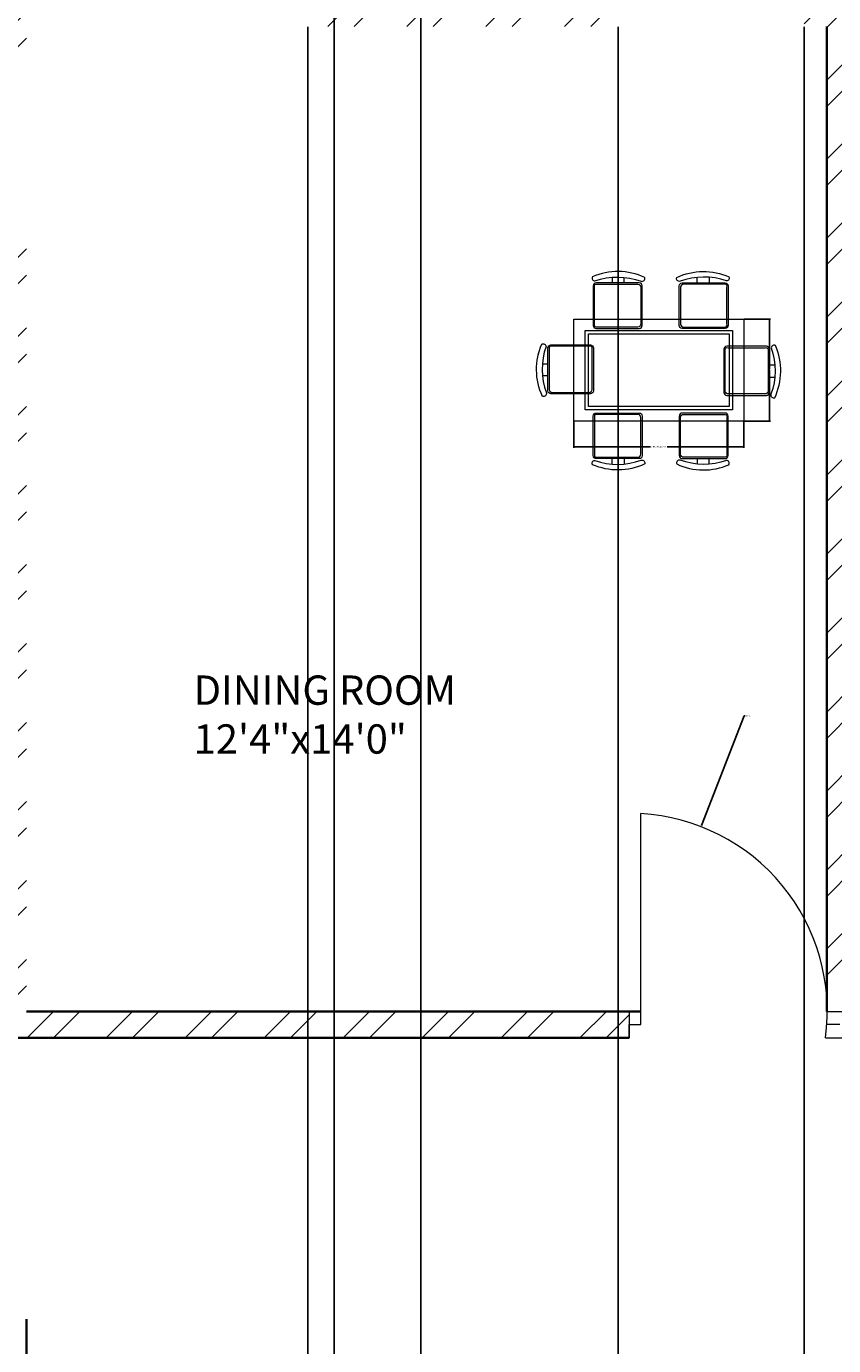
# Model space of a CAD drawing. Units: inches. Extents: x 392 to 1254, y 1207 to 2665.
# Tile 7 of 15: x 694 to 832, y 1827 to 2052. Entities that reach past the tile are written whole.
import ezdxf

# ---------------------------------------------------------------- set-up
doc = ezdxf.new("R2010")
doc.units = ezdxf.units.IN
for name, color, linetype, lineweight in [('A-ANNO-DIMS', 2, 'Continuous', 18), ('A-AREA-IDEN', 7, 'Continuous', 18), ('A-DOOR', 3, 'Continuous', 18), ('A-FURN', 8, 'Continuous', 13), ('A-WALL', 7, 'Continuous', 35), ('A-WALL-PATT', 252, 'Continuous', 13)]:
    doc.layers.add(name, color=color, linetype=linetype, lineweight=lineweight)
doc.styles.get("Standard").update_dxf_attribs({"font": 'arial.ttf'})
doc.dimstyles.get("Standard").update_dxf_attribs({"dimtxt": 0.18, "dimasz": 0.18, "dimexe": 0.18, "dimexo": 0.0625, "dimgap": 0.09, "dimtad": 0, "dimtih": 1, "dimtoh": 1, "dimdec": 4, "dimzin": 0, "dimdsep": 46, "dimtxsty": 'Standard', "dimcen": 0.09, "dimadec": 0, "dimazin": 0, "dimtfac": 1, "dimtdec": 4, "dimtofl": 0, "dimtmove": 0, "dimatfit": 3, "dimfxl": 1, "dimtolj": 1, "dimtzin": 0, "dimarcsym": 0})

# ---------------------------------------------------------------- blocks, each defined once
blk = doc.blocks.new('TABLE-DINING-RECT')
for points in [[(0, 17.41), (29.01, 17.41), (29.01, 0), (0, 0)], [(0, 17.41), (29.01, 17.41), (29.01, 0), (0, 0)], [(1.93, 15.47), (27.08, 15.47), (27.08, 1.93), (1.93, 1.93)], [(1.93, 15.47), (27.08, 15.47), (27.08, 1.93), (1.93, 1.93)], [(2.51, 14.89), (26.5, 14.89), (26.5, 2.51), (2.51, 2.51)], [(2.51, 14.89), (26.5, 14.89), (26.5, 2.51), (2.51, 2.51)]]:
    blk.add_lwpolyline(points, close=True)
blk = doc.blocks.new('*D19')
at = {"layer": 'A-ANNO-DIMS', "color": 0, "lineweight": -2, "transparency": 16777216}
for p, q in [((787.64, 1984.9), (787.64, 1980.43)), ((816.65, 1984.9), (816.65, 1980.43)), ((787.82, 1980.61), (800.71, 1980.61)), ((816.47, 1980.61), (803.58, 1980.61))]:
    blk.add_line(p, q, dxfattribs=at)
at = {"layer": 'A-ANNO-DIMS', "color": 0, "transparency": 16777216}
for points in [[(787.82, 1980.64), (787.82, 1980.58), (787.64, 1980.61)], [(816.47, 1980.64), (816.47, 1980.58), (816.65, 1980.61)]]:
    blk.add_solid(points, dxfattribs=at)
at = {"layer": 'Defpoints', "color": 0, "transparency": 16777216}
for p in [(787.64, 1984.96), (816.65, 1984.96), (816.65, 1980.61)]:
    blk.add_point(p, dxfattribs=at)
at = {"layer": 'A-ANNO-DIMS', "color": 0, "transparency": 16777216, "insert": (802.15, 1980.61), "char_height": 0.18, "attachment_point": 5}
blk.add_mtext('\\A1;DINING TABLE 29 TYP.', dxfattribs=at)
blk = doc.blocks.new('*D20')
at = {"layer": 'A-ANNO-DIMS', "color": 0, "lineweight": -2, "transparency": 16777216}
for p, q in [((816.71, 2002.37), (821.18, 2002.37)), ((821, 2002.19), (821, 1993.84)), ((821, 1985.14), (821, 1993.48)), ((816.71, 1984.96), (821.18, 1984.96))]:
    blk.add_line(p, q, dxfattribs=at)
at = {"layer": 'A-ANNO-DIMS', "color": 0, "transparency": 16777216}
for points in [[(820.97, 2002.19), (821.03, 2002.19), (821, 2002.37)], [(820.97, 1985.14), (821.03, 1985.14), (821, 1984.96)]]:
    blk.add_solid(points, dxfattribs=at)
at = {"layer": 'Defpoints', "color": 0, "transparency": 16777216}
for p in [(816.65, 2002.37), (821, 2002.37), (816.65, 1984.96)]:
    blk.add_point(p, dxfattribs=at)
at = {"layer": 'A-ANNO-DIMS', "color": 0, "transparency": 16777216, "insert": (821, 1993.66), "char_height": 0.18, "attachment_point": 5}
blk.add_mtext('\\A1;17 TYP.', dxfattribs=at)
blk = doc.blocks.new('*D26')
at = {"layer": 'A-ANNO-DIMS', "color": 0, "lineweight": -2, "transparency": 16777216}
for p, q in [((541.22, 2229.3), (495, 2229.3)), ((495.18, 2229.12), (495.18, 1819.98)), ((495.18, 1410.48), (495.18, 1819.61)), ((753.23, 1410.3), (495, 1410.3))]:
    blk.add_line(p, q, dxfattribs=at)
at = {"layer": 'A-ANNO-DIMS', "color": 0, "transparency": 16777216}
for points in [[(495.15, 2229.12), (495.21, 2229.12), (495.18, 2229.3)], [(495.15, 1410.48), (495.21, 1410.48), (495.18, 1410.3)]]:
    blk.add_solid(points, dxfattribs=at)
at = {"layer": 'Defpoints', "color": 0, "transparency": 16777216}
for p in [(495.18, 2229.3), (541.28, 2229.3), (753.29, 1410.3)]:
    blk.add_point(p, dxfattribs=at)
at = {"layer": 'A-ANNO-DIMS', "color": 0, "transparency": 16777216, "insert": (495.18, 1819.8), "char_height": 0.18, "attachment_point": 5}
blk.add_mtext('\\A1;819', dxfattribs=at)
blk = doc.blocks.new('*D75')
at = {"layer": 'A-ANNO-DIMS', "color": 0, "lineweight": -2, "transparency": 16777216}
for p, q in [((746.78, 2056.73), (746.78, 1364.02)), ((742.28, 2052.23), (742.28, 1364.02)), ((742.46, 1364.2), (744.27, 1364.2)), ((746.6, 1364.2), (744.79, 1364.2))]:
    blk.add_line(p, q, dxfattribs=at)
at = {"layer": 'A-ANNO-DIMS', "color": 0, "transparency": 16777216}
for points in [[(742.46, 1364.23), (742.46, 1364.17), (742.28, 1364.2)], [(746.6, 1364.23), (746.6, 1364.17), (746.78, 1364.2)]]:
    blk.add_solid(points, dxfattribs=at)
at = {"layer": 'Defpoints', "color": 0, "transparency": 16777216}
for p in [(746.78, 2056.8), (742.28, 2052.3), (746.78, 1364.2)]:
    blk.add_point(p, dxfattribs=at)
at = {"layer": 'A-ANNO-DIMS', "color": 0, "transparency": 16777216, "insert": (744.53, 1364.2), "char_height": 0.18, "attachment_point": 5}
blk.add_mtext('\\A1;4.5', dxfattribs=at)
blk = doc.blocks.new('*D78')
at = {"layer": 'A-ANNO-DIMS', "color": 0, "lineweight": -2, "transparency": 16777216}
for p, q in [((746.78, 2056.73), (746.78, 1364.02)), ((761.56, 2056.73), (761.56, 1364.02)), ((746.96, 1364.2), (753.72, 1364.2)), ((761.38, 1364.2), (754.63, 1364.2))]:
    blk.add_line(p, q, dxfattribs=at)
at = {"layer": 'A-ANNO-DIMS', "color": 0, "transparency": 16777216}
for points in [[(746.96, 1364.23), (746.96, 1364.17), (746.78, 1364.2)], [(761.38, 1364.23), (761.38, 1364.17), (761.56, 1364.2)]]:
    blk.add_solid(points, dxfattribs=at)
at = {"layer": 'Defpoints', "color": 0, "transparency": 16777216}
for p in [(746.78, 2056.8), (761.56, 2056.8), (761.56, 1364.2)]:
    blk.add_point(p, dxfattribs=at)
at = {"layer": 'A-ANNO-DIMS', "color": 0, "transparency": 16777216, "insert": (754.17, 1364.2), "char_height": 0.18, "attachment_point": 5}
blk.add_mtext('\\A1;14.782', dxfattribs=at)
blk = doc.blocks.new('*D80')
at = {"layer": 'A-ANNO-DIMS', "color": 0, "lineweight": -2, "transparency": 16777216}
for p, q in [((795.21, 2052.23), (795.21, 1364.02)), ((826.91, 2052.23), (826.91, 1364.02)), ((795.39, 1364.2), (810.6, 1364.2)), ((826.73, 1364.2), (811.52, 1364.2))]:
    blk.add_line(p, q, dxfattribs=at)
at = {"layer": 'A-ANNO-DIMS', "color": 0, "transparency": 16777216}
for points in [[(795.39, 1364.23), (795.39, 1364.17), (795.21, 1364.2)], [(826.73, 1364.23), (826.73, 1364.17), (826.91, 1364.2)]]:
    blk.add_solid(points, dxfattribs=at)
at = {"layer": 'Defpoints', "color": 0, "transparency": 16777216}
for p in [(795.21, 2052.3), (826.91, 2052.3), (826.91, 1364.2)]:
    blk.add_point(p, dxfattribs=at)
at = {"layer": 'A-ANNO-DIMS', "color": 0, "transparency": 16777216, "insert": (811.06, 1364.2), "char_height": 0.18, "attachment_point": 5}
blk.add_mtext('\\A1;31.694', dxfattribs=at)
blk = doc.blocks.new('*D83')
at = {"layer": 'A-ANNO-DIMS', "color": 0, "lineweight": -2, "transparency": 16777216}
for p, q in [((816.68, 1934.68), (809.41, 1915.98)), ((816.86, 1934.68), (816.68, 1934.68)), ((797.03, 1884.36), (797.21, 1884.36)), ((797.12, 1884.27), (797.12, 1884.45))]:
    blk.add_line(p, q, dxfattribs=at)
at = {"layer": 'A-ANNO-DIMS', "color": 0, "transparency": 16777216}
blk.add_solid([(809.38, 1915.99), (809.44, 1915.97), (809.34, 1915.81)], dxfattribs=at)
at = {"layer": 'Defpoints', "color": 0, "transparency": 16777216}
for p in [(809.34, 1915.81), (797.12, 1884.36)]:
    blk.add_point(p, dxfattribs=at)
at = {"layer": 'A-ANNO-DIMS', "color": 0, "transparency": 16777216, "insert": (817.34, 1934.68), "char_height": 0.18, "attachment_point": 5}
blk.add_mtext('\\A1;R33.74', dxfattribs=at)

msp = doc.modelspace()

# ---------------------------------------------------------------- hatches: boundary and pattern name
at = {"layer": 'A-WALL-PATT'}
h = msp.add_hatch(dxfattribs=at)
h.set_pattern_fill('ANSI32', color=256)
h.paths.add_polyline_path([(579.5309, 2227.0453), (579.5309, 2229.2953), (541.2807, 2229.2953), (541.2807, 2182.3091), (545.7807, 2182.3091), (545.7807, 2224.7953), (579.5309, 2224.7953)])
h.paths.add_polyline_path([(655.4442, 2229.2953), (627.5309, 2229.2953), (627.5309, 2224.7953), (655.4442, 2224.7953), (655.4442, 2227.0453)])
h.paths.add_polyline_path([(703.0758, 2229.2953), (678.5257, 2229.2953), (678.5257, 2227.0453), (678.5257, 2224.7953), (689.7807, 2224.7953), (689.7807, 2158.6973), (694.2807, 2158.6973), (694.2807, 2224.7953), (703.0758, 2224.7953)])
h.paths.add_polyline_path([(768.5767, 2229.2953), (727.0758, 2229.2953), (727.0758, 2224.7953), (742.2807, 2224.7953), (742.2807, 2128.7953), (694.2807, 2128.7953), (694.2807, 2134.0554), (689.7807, 2134.0554), (689.7807, 2090.2854), (694.2807, 2090.2854), (694.2807, 2124.2953), (742.2807, 2124.2953), (742.2807, 2052.2953), (795.2123, 2052.2953), (795.2123, 2054.5453), (795.2123, 2056.7953), (746.7807, 2056.7953), (746.7807, 2224.7953), (768.5767, 2224.7953)])
h.paths.add_polyline_path([(867.5089, 2229.2953), (804.5767, 2229.2953), (804.5767, 2224.7953), (830.7807, 2224.7953), (830.7807, 2056.7953), (826.9066, 2056.7953), (826.9066, 2052.2953), (830.7807, 2052.2953), (830.7807, 1886.6777, -0.01766664), (830.8602, 1884.2953), (835.0818, 1884.2953, -0.04411348), (835.2807, 1889.9369), (835.2807, 2052.2953), (839.418, 2052.2953), (839.418, 2056.7953), (835.2807, 2056.7953), (835.2807, 2224.7953), (867.5089, 2224.7953)])
h.paths.add_polyline_path([(939.8604, 2229.2953), (903.5089, 2229.2953), (903.5089, 2227.0453), (903.5089, 2224.7953), (919.2807, 2224.7953), (919.2807, 2056.7953), (870.6499, 2056.7953), (870.6499, 2052.2953), (923.7807, 2052.2953), (923.7807, 2124.2953), (971.7807, 2124.2953), (971.7807, 2089.7112), (974.0307, 2089.7112), (976.2807, 2089.7112), (976.2807, 2133.56), (974.0307, 2133.56), (971.7807, 2133.56), (971.7807, 2128.7953), (923.7807, 2128.7953), (923.7807, 2224.7953), (939.8604, 2224.7953)])
h.paths.add_polyline_path([(1124.7807, 2229.2953), (1009.403, 2229.2953), (1009.403, 2224.7953), (1120.2807, 2224.7953), (1120.2807, 2184.7605), (1124.7807, 2184.7605)])
h.paths.add_polyline_path([(1124.7807, 2124.7605), (1120.2807, 2124.7605), (1120.2807, 2056.7953), (976.2807, 2056.7953), (976.2807, 2061.471), (971.7807, 2061.471), (971.7807, 2047.7483), (974.0307, 2047.7483), (976.2807, 2047.7483), (976.2807, 2052.2953), (1120.2807, 2052.2953), (1120.2807, 1992.457), (1124.7807, 1992.457)])
h.paths.add_polyline_path([(1124.7807, 1932.457), (1122.5307, 1932.457), (1120.2807, 1932.457), (1120.2807, 1884.2953), (976.2807, 1884.2953), (976.2807, 2019.9536), (971.7807, 2019.9536), (971.7807, 1884.2953), (869.0911, 1884.2953), (869.0911, 1879.7953), (971.7807, 1879.7953), (1013.7807, 1879.7953), (1013.7807, 1831.7953), (971.7807, 1831.7953), (971.7807, 1822.3831), (974.0307, 1822.3831), (976.2807, 1822.3831), (976.2807, 1827.2953), (1013.7807, 1827.2953), (1025.6191, 1827.2953), (1025.6191, 1829.5453), (1025.6191, 1831.7953), (1018.2807, 1831.7953), (1018.2807, 1879.7953), (1120.2807, 1879.7953), (1120.2807, 1866.9192), (1124.7807, 1866.9192)])
h.paths.add_polyline_path([(1124.7807, 1842.9192), (1122.5307, 1842.9192), (1120.2807, 1842.9192), (1120.2807, 1831.7953), (1050.2021, 1831.7953), (1050.2021, 1827.2953), (1120.2807, 1827.2953), (1120.2807, 1781.4559), (1124.7807, 1781.4559)])
h.paths.add_polyline_path([(976.2807, 1790.8718), (971.7807, 1790.8718), (971.7807, 1648.3339), (976.2807, 1648.3339), (976.2807, 1654.7953), (1120.2807, 1654.7953), (1120.2807, 1626.3807), (1124.7807, 1626.3807), (1124.7807, 1721.4559), (1120.2807, 1721.4559), (1120.2807, 1659.2953), (976.2807, 1659.2953)])
h.paths.add_polyline_path([(1124.7807, 1566.3807), (1120.2807, 1566.3807), (1120.2807, 1486.7953), (1101.07, 1486.7953), (1101.07, 1482.2953), (1124.7807, 1482.2953)])
h.paths.add_polyline_path([(1041.07, 1484.5453), (1041.07, 1486.7953), (1006.2807, 1486.7953), (1006.2807, 1484.5453), (1006.2807, 1482.2953), (1041.07, 1482.2953)])
h.paths.add_polyline_path([(976.2807, 1617.5497), (974.0307, 1617.5497), (971.7807, 1617.5497), (971.7807, 1599.2953), (965.8041, 1599.2953), (965.8041, 1594.7953), (971.7807, 1594.7953), (971.7807, 1486.7953), (954.1249, 1486.7953), (954.1249, 1482.2953), (981.5717, 1482.2953), (981.5717, 1484.5453), (981.5717, 1486.7953), (976.2807, 1486.7953)])
h.paths.add_polyline_path([(930.1249, 1486.7953), (887.7807, 1486.7953), (887.7807, 1594.7953), (941.9141, 1594.7953), (941.9141, 1597.0453), (941.9141, 1599.2953), (887.7807, 1599.2953), (887.7807, 1659.2953), (863.5916, 1659.2953), (863.5916, 1654.7953), (883.2807, 1654.7953), (883.2807, 1438.7953), (782.7807, 1438.7953), (782.7807, 1486.7953), (782.7807, 1654.7953), (800.1309, 1654.7953), (800.1309, 1657.0453), (800.1309, 1659.2953), (778.2807, 1659.2953), (778.2807, 1599.2953), (721.7333, 1599.2953), (721.7333, 1597.0453), (721.7333, 1594.7953), (778.2807, 1594.7953), (778.2807, 1486.7953), (729.598, 1486.7953), (729.598, 1482.2953), (753.2885, 1482.2953), (753.2885, 1410.2953), (922.9852, 1410.2953), (922.9852, 1482.2953), (930.1249, 1482.2953)])
h.paths.add_polyline_path([(918.4852, 1482.2953), (918.4852, 1414.7953), (757.7885, 1414.7953), (757.7885, 1482.2953), (778.2807, 1482.2953), (778.2807, 1434.2953), (782.7807, 1434.2953), (887.7807, 1434.2953), (887.7807, 1438.7953), (887.7807, 1482.2953)], flags=16)
h.paths.add_polyline_path([(694.2807, 1594.7953), (700.4169, 1594.7953), (700.4169, 1597.0453), (700.4169, 1599.2953), (694.2807, 1599.2953), (694.2807, 1617.7503), (692.0307, 1617.7503), (689.7807, 1617.7503), (689.7807, 1486.7953), (682.7672, 1486.7953), (682.7672, 1482.2953), (705.598, 1482.2953), (705.598, 1484.5453), (705.598, 1486.7953), (694.2807, 1486.7953)])
h.paths.add_polyline_path([(545.7807, 1654.7953), (689.7807, 1654.7953), (689.7807, 1649.7691), (694.2807, 1649.7691), (694.2807, 1789.3981), (692.0307, 1789.3981), (689.7807, 1789.3981), (689.7807, 1659.2953), (545.7807, 1659.2953), (545.7807, 1714.4681), (543.5307, 1714.4681), (541.2807, 1714.4681), (541.2807, 1482.2953), (567.0628, 1482.2953), (567.0628, 1484.5453), (567.0628, 1486.7953), (545.7807, 1486.7953)])
h.paths.add_polyline_path([(545.7807, 1827.2953), (620.2247, 1827.2953), (620.2247, 1829.5453), (620.2247, 1831.7953), (545.7807, 1831.7953), (545.7807, 1846.8518), (541.2807, 1846.8518), (541.2807, 1774.4681), (545.7807, 1774.4681)])
h.paths.add_polyline_path([(797.0944, 1884.2953), (694.2807, 1884.2953), (694.2807, 2019.0288), (692.0307, 2019.0288), (689.7807, 2019.0288), (689.7807, 1884.2953), (545.7807, 1884.2953), (545.7807, 1951.8244), (541.2807, 1951.8244), (541.2807, 1870.8518), (543.5307, 1870.8518), (545.7807, 1870.8518), (545.7807, 1879.7953), (647.7807, 1879.7953), (647.7807, 1831.7953), (642.6413, 1831.7953), (642.6413, 1827.2953), (652.2807, 1827.2953), (689.7807, 1827.2953), (689.7807, 1821.0531), (694.2807, 1821.0531), (694.2807, 1831.7953), (652.2807, 1831.7953), (652.2807, 1879.7953), (797.0944, 1879.7953), (797.0944, 1882.0453)])
h.paths.add_polyline_path([(545.7807, 2122.3091), (541.2807, 2122.3091), (541.2807, 2011.8244), (543.5307, 2011.8244), (545.7807, 2011.8244), (545.7807, 2052.2953), (689.7807, 2052.2953), (689.7807, 2048.2048), (694.2807, 2048.2048), (694.2807, 2061.3129), (692.0307, 2061.3129), (689.7807, 2061.3129), (689.7807, 2056.7953), (545.7807, 2056.7953)])

# ---------------------------------------------------------------- linework, layer by layer
at = {"layer": 'A-DOOR'}
for p, q in [((799.0944, 1882.0453), (799.0944, 1918.0453)), ((797.0944, 1884.2953), (797.0944, 1879.7953)), ((830.7807, 1884.2953), (835.0818, 1884.2953)), ((797.0944, 1879.7953), (797.0944, 1882.0453)), ((797.0944, 1882.0453), (799.0944, 1882.0453)), ((833.0352, 1882.0453), (830.7807, 1882.0453)), ((830.5499, 1879.7953), (835.2807, 1879.7953))]:
    msp.add_line(p, q, dxfattribs=at)
msp.add_arc((797.1186, 1884.3615), 33.7417, 352.222464, 86.64301, dxfattribs=at)
at = {"layer": 'A-FURN'}
for points in [[(791.2286, 2008.878, -0.17580919), (799.1303, 2008.8182, 0.57839206), (799.729, 2009.4764, 0.21452438), (790.8096, 2009.5961, 0.55201397), (791.2286, 2008.878, -0.06507904)], [(791.2287, 2008.8777, -0.17580919), (799.1304, 2008.8179, 0.57839206), (799.729, 2009.4761, 0.21452438), (790.8096, 2009.5958, 0.55201397), (791.2287, 2008.8777, -0.06507904)], [(796.2184, 2008.5609), (796.2184, 2009.4886, -0.06475861)], [(796.2185, 2008.5606), (796.2185, 2009.4883, -0.06475861)], [(805.7826, 2008.8182, -0.57839206), (805.1839, 2009.4764, -0.21452438), (814.1033, 2009.5961, -0.55201397), (813.6843, 2008.878, 0.1758092), (805.7826, 2008.8182)], [(805.7826, 2008.8179, -0.57839206), (805.184, 2009.4761, -0.21452438), (814.1033, 2009.5958, -0.55201397), (813.6843, 2008.8777, 0.1758092), (805.7826, 2008.8179)], [(808.6944, 2008.5609), (808.6944, 2009.4886, 0.06475861)], [(808.6945, 2008.5606), (808.6945, 2009.4883, 0.06475861)], [(798.7951, 2008.5609), (791.4594, 2008.5609, 0.41421356), (790.9462, 2008.0477), (790.9462, 2001.3027, 0.41421356), (791.4594, 2000.7894), (798.7951, 2000.7894, 0.41421356), (799.3083, 2001.3027), (799.3083, 2008.0477, 0.41421356), (798.7951, 2008.5609)], [(798.7951, 2008.5606), (791.4594, 2008.5606, 0.41421356), (790.9462, 2008.0474), (790.9462, 2001.3023, 0.41421356), (791.4594, 2000.7891), (798.7951, 2000.7891, 0.41421356), (799.3083, 2001.3023), (799.3083, 2008.0474, 0.41421356), (798.7951, 2008.5606)], [(813.4535, 2008.5609, -0.41421356), (813.9667, 2008.0477), (813.9667, 2001.3027, -0.41421356), (813.4535, 2000.7894), (806.1178, 2000.7894, -0.41421356), (805.6046, 2001.3027), (805.6046, 2008.0477, -0.41421356), (806.1178, 2008.5609), (813.4535, 2008.5609)], [(813.4535, 2008.5606, -0.41421356), (813.9667, 2008.0474), (813.9667, 2001.3023, -0.41421356), (813.4535, 2000.7891), (806.1178, 2000.7891, -0.41421356), (805.6046, 2001.3023), (805.6046, 2008.0474, -0.41421356), (806.1178, 2008.5606), (813.4535, 2008.5606)], [(782.9619, 1989.7966, -0.57839206), (782.3037, 1989.198, -0.21452438), (782.184, 1998.1173, -0.55201397), (782.9021, 1997.6983, 0.17580937), (782.9619, 1989.7966)], [(782.962, 1989.7963, -0.57839206), (782.3037, 1989.1977, -0.21452438), (782.1841, 1998.117, -0.55201397), (782.9021, 1997.698, 0.17580937), (782.962, 1989.7963)], [(783.2192, 1997.4675, -0.41421356), (783.7325, 1997.9807), (790.4775, 1997.9807, -0.41421356), (790.9907, 1997.4675), (790.9907, 1990.1318, -0.41421356), (790.4775, 1989.6186), (783.7325, 1989.6186, -0.41421356), (783.2192, 1990.1318), (783.2192, 1997.4675)], [(783.2193, 1997.4672, -0.41421356), (783.7325, 1997.9804), (790.4775, 1997.9804, -0.41421356), (790.9907, 1997.4672), (790.9907, 1990.1315, -0.41421356), (790.4775, 1989.6183), (783.7325, 1989.6183, -0.41421356), (783.2193, 1990.1315), (783.2193, 1997.4672)], [(820.9945, 1997.2163, 0.41421356), (820.4813, 1997.7295), (813.7363, 1997.7295, 0.41421356), (813.2231, 1997.2163), (813.2231, 1989.8806, 0.41421356), (813.7363, 1989.3674), (820.4813, 1989.3674, 0.41421356), (820.9945, 1989.8806), (820.9945, 1997.2163)], [(820.9945, 1997.216, 0.41421356), (820.4813, 1997.7292), (813.7363, 1997.7292, 0.41421356), (813.2231, 1997.216), (813.2231, 1989.8803, 0.41421356), (813.7363, 1989.3671), (820.4813, 1989.3671, 0.41421356), (820.9945, 1989.8803), (820.9945, 1997.216)], [(821.3117, 1997.4471, -0.17580919), (821.2518, 1989.5454, 0.57839206), (821.91, 1988.9468, 0.21452438), (822.0297, 1997.8661, 0.55201397), (821.3117, 1997.4471, -0.06507904)], [(821.3117, 1997.4468, -0.17580919), (821.2518, 1989.5451, 0.57839206), (821.9101, 1988.9464, 0.21452438), (822.0297, 1997.8658, 0.55201397), (821.3117, 1997.4468, -0.06507904)], [(783.2192, 1992.7085), (782.2915, 1992.7085, 0.06475861)], [(783.2193, 1992.7082), (782.2915, 1992.7082, 0.06475861)], [(820.9945, 1992.4573), (821.9223, 1992.4573, -0.06475861)], [(820.9945, 1992.457), (821.9223, 1992.457, -0.06475861)], [(798.7951, 1978.5777), (791.4594, 1978.5777, -0.41421356), (790.9462, 1979.0909), (790.9462, 1985.8359, -0.41421356), (791.4594, 1986.3491), (798.7951, 1986.3491, -0.41421356), (799.3083, 1985.8359), (799.3083, 1979.0909, -0.41421356), (798.7951, 1978.5777)], [(798.7951, 1978.5773), (791.4594, 1978.5773, -0.41421356), (790.9462, 1979.0906), (790.9462, 1985.8356, -0.41421356), (791.4594, 1986.3488), (798.7951, 1986.3488, -0.41421356), (799.3083, 1985.8356), (799.3083, 1979.0906, -0.41421356), (798.7951, 1978.5773)], [(813.4535, 1978.5777, 0.41421356), (813.9667, 1979.0909), (813.9667, 1985.8359, 0.41421356), (813.4535, 1986.3491), (806.1178, 1986.3491, 0.41421356), (805.6046, 1985.8359), (805.6046, 1979.0909, 0.41421356), (806.1178, 1978.5777), (813.4535, 1978.5777)], [(813.4535, 1978.5773, 0.41421356), (813.9667, 1979.0906), (813.9667, 1985.8356, 0.41421356), (813.4535, 1986.3488), (806.1178, 1986.3488, 0.41421356), (805.6046, 1985.8356), (805.6046, 1979.0906, 0.41421356), (806.1178, 1978.5773), (813.4535, 1978.5773)], [(799.1303, 1978.3204, -0.57839206), (799.729, 1977.6621, -0.21452438), (790.8096, 1977.5425, -0.55201397), (791.2286, 1978.2605, 0.17580929), (799.1303, 1978.3204)], [(799.1304, 1978.32, -0.57839206), (799.729, 1977.6618, -0.21452438), (790.8096, 1977.5421, -0.55201397), (791.2287, 1978.2602, 0.17580929), (799.1304, 1978.32)], [(796.2184, 1978.5777), (796.2184, 1977.6499, 0.06475861)], [(796.2185, 1978.5773), (796.2185, 1977.6496, 0.06475861)], [(813.6843, 1978.2605, -0.17580928), (805.7826, 1978.3204, 0.57839206), (805.1839, 1977.6621, 0.21452438), (814.1033, 1977.5425, 0.55201397), (813.6843, 1978.2605, -0.06507904)], [(813.6843, 1978.2602, -0.17580928), (805.7826, 1978.32, 0.57839206), (805.184, 1977.6618, 0.21452438), (814.1033, 1977.5421, 0.55201397), (813.6843, 1978.2602, -0.06507904)], [(808.6944, 1978.5777), (808.6944, 1977.6499, -0.06475861)], [(808.6945, 1978.5773), (808.6945, 1977.6496, -0.06475861)]]:
    msp.add_lwpolyline(points, format="xyb", dxfattribs=at)
for points in [[(794.1651, 2009.5055), (794.1651, 2008.5609)], [(794.1651, 2009.5052), (794.1651, 2008.5606)], [(810.7478, 2009.5055), (810.7478, 2008.5609)], [(810.7478, 2009.5052), (810.7478, 2008.5606)], [(782.2746, 1994.7619), (783.2192, 1994.7619)], [(782.2747, 1994.7616), (783.2193, 1994.7616)], [(821.9391, 1994.5106), (820.9945, 1994.5106)], [(821.9391, 1994.5103), (820.9945, 1994.5103)], [(794.1651, 1977.6331), (794.1651, 1978.5777)], [(794.1651, 1977.6328), (794.1651, 1978.5773)], [(810.7478, 1977.6331), (810.7478, 1978.5777)], [(810.7478, 1977.6328), (810.7478, 1978.5773)]]:
    msp.add_lwpolyline(points, dxfattribs=at)
for points in [[(791.4625, 2008.3297), (798.5639, 2008.3297, -0.41421356), (799.0771, 2007.8165), (799.0771, 2001.5339, -0.41421356), (798.5639, 2001.0206), (791.4625, 2001.0206, -0.51206948), (791.1774, 2001.5339), (791.1774, 2007.8165, -0.51206948)], [(791.4626, 2008.3294), (798.5639, 2008.3294, -0.41421356), (799.0771, 2007.8162), (799.0771, 2001.5336, -0.41421356), (798.5639, 2001.0203), (791.4626, 2001.0203, -0.51206948), (791.1774, 2001.5336), (791.1774, 2007.8162, -0.51206948)], [(813.4503, 2008.3297), (806.349, 2008.3297, 0.41421356), (805.8358, 2007.8165), (805.8358, 2001.5339, 0.41421356), (806.349, 2001.0206), (813.4503, 2001.0206, 0.51206948), (813.7355, 2001.5339), (813.7355, 2007.8165, 0.51206948)], [(813.4504, 2008.3294), (806.349, 2008.3294, 0.41421356), (805.8358, 2007.8162), (805.8358, 2001.5336, 0.41421356), (806.349, 2001.0203), (813.4504, 2001.0203, 0.51206948), (813.7355, 2001.5336), (813.7355, 2007.8162, 0.51206948)], [(783.4504, 1997.4644), (783.4504, 1990.363, 0.41421356), (783.9637, 1989.8498), (790.2463, 1989.8498, 0.41421356), (790.7595, 1990.363), (790.7595, 1997.4644, 0.51206948), (790.2463, 1997.7495), (783.9637, 1997.7495, 0.51206948)], [(783.4505, 1997.4641), (783.4505, 1990.3627, 0.41421356), (783.9637, 1989.8495), (790.2463, 1989.8495, 0.41421356), (790.7595, 1990.3627), (790.7595, 1997.4641, 0.51206948), (790.2463, 1997.7492), (783.9637, 1997.7492, 0.51206948)], [(820.7633, 1997.2132), (820.7633, 1990.1118, -0.41421356), (820.2501, 1989.5986), (813.9675, 1989.5986, -0.41421356), (813.4543, 1990.1118), (813.4543, 1997.2132, -0.51206948), (813.9675, 1997.4983), (820.2501, 1997.4983, -0.51206948)], [(820.7633, 1997.2129), (820.7633, 1990.1115, -0.41421356), (820.2501, 1989.5983), (813.9675, 1989.5983, -0.41421356), (813.4543, 1990.1115), (813.4543, 1997.2129, -0.51206948), (813.9675, 1997.498), (820.2501, 1997.498, -0.51206948)], [(791.4625, 1978.8089), (798.5639, 1978.8089, 0.41421356), (799.0771, 1979.3221), (799.0771, 1985.6047, 0.41421356), (798.5639, 1986.1179), (791.4625, 1986.1179, 0.51206948), (791.1774, 1985.6047), (791.1774, 1979.3221, 0.51206948)], [(791.4626, 1978.8086), (798.5639, 1978.8086, 0.41421356), (799.0771, 1979.3218), (799.0771, 1985.6044, 0.41421356), (798.5639, 1986.1176), (791.4626, 1986.1176, 0.51206948), (791.1774, 1985.6044), (791.1774, 1979.3218, 0.51206948)], [(813.4503, 1978.8089), (806.349, 1978.8089, -0.41421356), (805.8358, 1979.3221), (805.8358, 1985.6047, -0.41421356), (806.349, 1986.1179), (813.4503, 1986.1179, -0.51206948), (813.7355, 1985.6047), (813.7355, 1979.3221, -0.51206948)], [(813.4504, 1978.8086), (806.349, 1978.8086, -0.41421356), (805.8358, 1979.3218), (805.8358, 1985.6044, -0.41421356), (806.349, 1986.1176), (813.4504, 1986.1176, -0.51206948), (813.7355, 1985.6044), (813.7355, 1979.3218, -0.51206948)]]:
    msp.add_lwpolyline(points, format="xyb", close=True, dxfattribs=at)
at = {"layer": 'A-WALL'}
for p, q in [((830.7807, 2052.2953), (830.7807, 1884.2953)), ((694.2807, 1884.2953), (799.0944, 1884.2953)), ((652.2807, 1879.7953), (797.0944, 1879.7953)), ((694.2807, 1831.7953), (694.2807, 1821.0531))]:
    msp.add_line(p, q, dxfattribs=at)

# ---------------------------------------------------------------- block references
at = {"layer": 'A-FURN'}
msp.add_blockref('TABLE-DINING-RECT', (787.64, 1984.959), dxfattribs=at)

# ---------------------------------------------------------------- texts
at = {"layer": 'A-AREA-IDEN', "insert": (722.7959, 1941.5918), "char_height": 5, "attachment_point": 1}
msp.add_mtext_dynamic_manual_height_columns('DINING ROOM\\P12\'4"x14\'0"', width=147.470137, gutter_width=12.5, heights=[0], dxfattribs=at)

# ---------------------------------------------------------------- dimensions: what is measured, and where the dimension line sits
at = {"layer": 'A-ANNO-DIMS'}
dim = msp.add_linear_dim(base=(495.1807, 2229.2953), p1=(753.2885, 1410.2953), p2=(541.2807, 2229.2953), angle=90, dimstyle='Standard', override={"dimdec": 0, "dimlfac": 1, "dimrnd": 0, "dimzin": 0, "dimdsep": 46, "dimlunit": 2}, dxfattribs=at)
dim.commit()
dim.dimension.update_dxf_attribs({"geometry": '*D26', "text_midpoint": (495.1807, 1819.7953)})
for base, p1, p2, override, picture, middle in [((746.7807, 1364.1953), (742.2807, 2052.2953), (746.7807, 2056.7953), {"dimdec": 1, "dimlfac": 1, "dimrnd": 0, "dimzin": 0, "dimdsep": 46, "dimlunit": 2}, '*D75', (744.5307, 1364.1953)), ((761.5625, 1364.1953), (746.7807, 2056.7953), (761.5625, 2056.7953), {"dimdec": 3, "dimlfac": 1, "dimrnd": 0, "dimzin": 0, "dimdsep": 46, "dimlunit": 2}, '*D78', (754.1716, 1364.1953)), ((826.9066, 1364.1953), (795.2123, 2052.2953), (826.9066, 2052.2953), {"dimdec": 3, "dimlfac": 1, "dimrnd": 0, "dimzin": 0, "dimdsep": 46, "dimlunit": 2}, '*D80', (811.0595, 1364.1953))]:
    dim = msp.add_linear_dim(base=base, p1=p1, p2=p2, dimstyle='Standard', override=override, dxfattribs=at)
    dim.commit()
    dim.dimension.update_dxf_attribs({"geometry": picture, "text_midpoint": middle})
dim = msp.add_linear_dim(base=(821.0027, 2002.3657), p1=(816.6511, 1984.959), p2=(816.6511, 2002.3657), angle=90, text='<> TYP.', dimstyle='Standard', override={"dimdec": 0, "dimlfac": 1, "dimrnd": 0, "dimzin": 0, "dimdsep": 46, "dimlunit": 2}, dxfattribs=at)
dim.commit()
dim.dimension.update_dxf_attribs({"geometry": '*D20', "text_midpoint": (821.0027, 1993.6623)})
dim = msp.add_linear_dim(base=(816.6511, 1980.6073), p1=(787.6403, 1984.959), p2=(816.6511, 1984.959), text='DINING TABLE <> TYP.', dimstyle='Standard', override={"dimdec": 0, "dimlfac": 1, "dimrnd": 0, "dimzin": 0, "dimdsep": 46, "dimlunit": 2}, dxfattribs=at)
dim.commit()
dim.dimension.update_dxf_attribs({"geometry": '*D19', "text_midpoint": (802.1457, 1980.6073)})
dim = msp.add_radius_dim(center=(797.1186, 1884.3615), mpoint=(809.3434, 1915.8108), dimstyle='Standard', override={"dimdec": 2, "dimlfac": 1, "dimrnd": 0, "dimzin": 0, "dimdsep": 46, "dimlunit": 2}, dxfattribs=at)
dim.commit()
dim.dimension.update_dxf_attribs({"geometry": '*D83', "text_midpoint": (817.3377, 1934.6804), "dimtype": 164})

doc.saveas('drawing.dxf')
